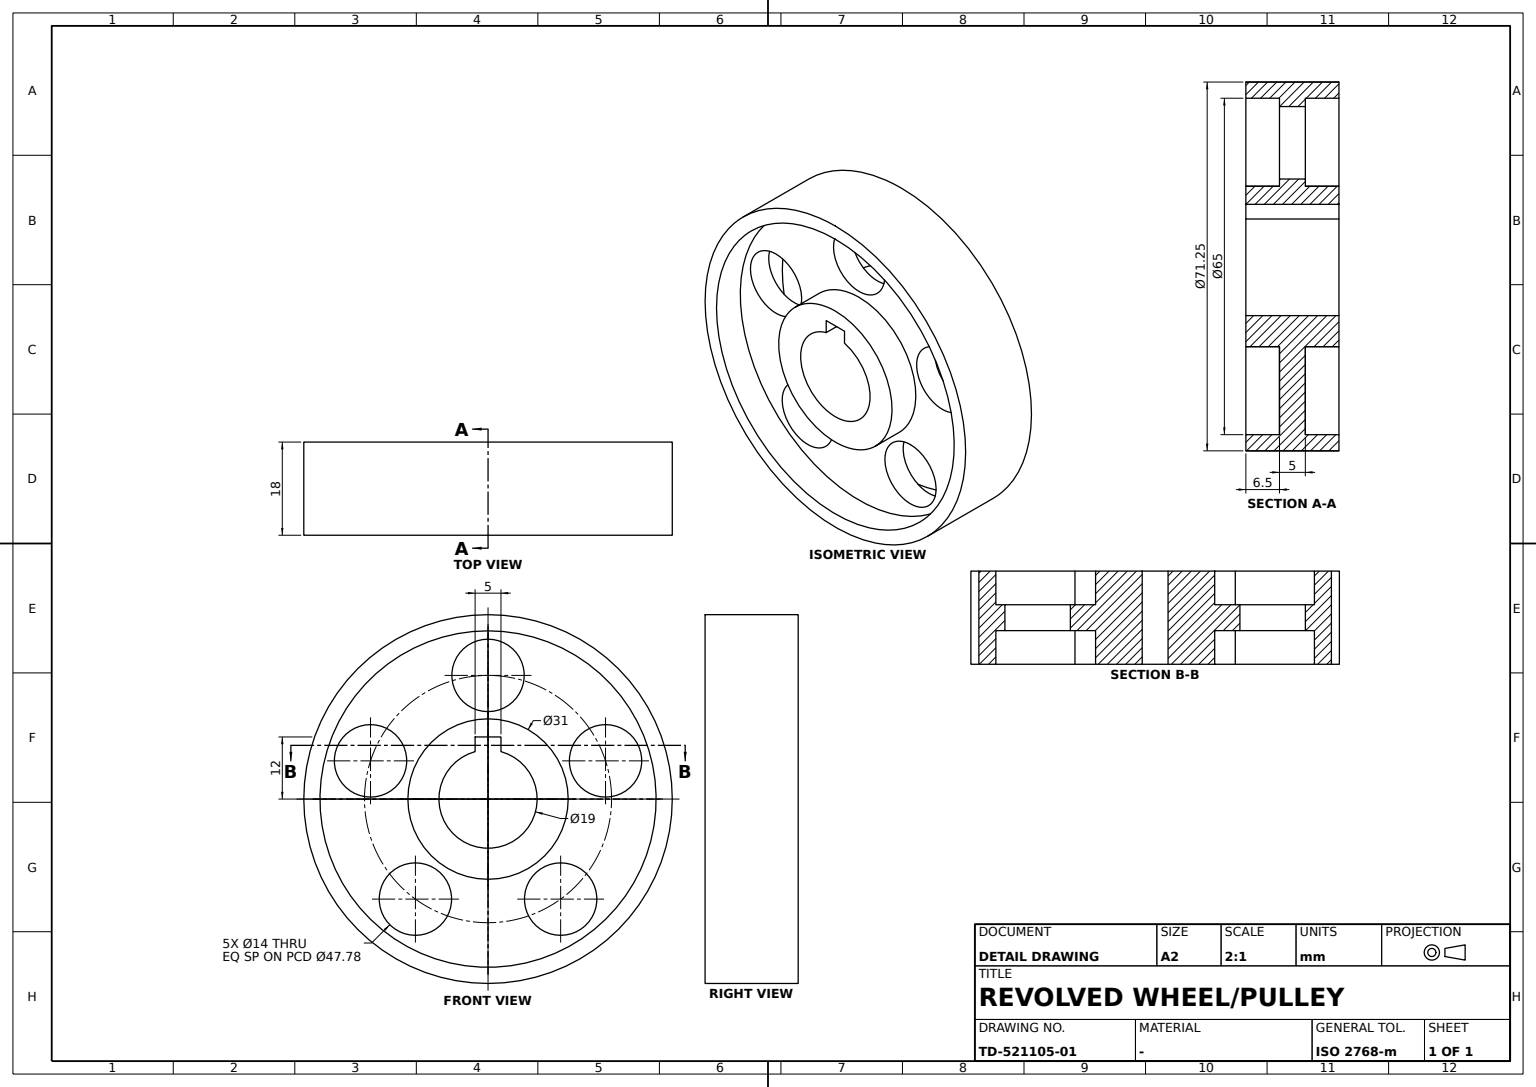
CATIA V5 part; units mm, degrees
sketch "Sketch1" plane through (0, 0, 0) normal (0, 1, 0) x (-1, 0, 0)
  point P0 (0, 9.5)
  line L0 (0, 9.5) -> (-5.7, 9.5)
  line L1 (-5.7, 9.5) -> (-5.7, 15.5)
  line L2 (-5.7, 15.5) -> (0.8, 15.5)
  line L3 (0.8, 15.5) -> (0.8, 32.5)
  line L4 (0.8, 32.5) -> (-5.7, 32.5)
  point P1 (-5.7, 32.5)
  line L5 (-5.7, 32.5) -> (-5.7, 35.625)
  point P2 (-5.7, 35.625)
  line L6 (-5.7, 35.625) -> (12.3, 35.625)
  line L7 (12.3, 35.625) -> (12.3, 32.5)
  point P3 (12.3, 32.5)
  line L8 (12.3, 32.5) -> (5.8, 32.5)
  line L9 (5.8, 32.5) -> (5.8, 15.5)
  point P4 (5.8, 15.5)
  line L10 (5.8, 15.5) -> (12.3, 15.5)
  point P5 (12.3, 15.5)
  line L11 (12.3, 15.5) -> (12.3, 9.5)
  point P6 (12.3, 9.5)
  line L12 (12.3, 9.5) -> (0, 9.5)
  dimension "length L7" = 3.125
  dimension "length L11" = 6
  dimension "distance L1 y axis" = 5.7
  dimension "distance L3 P2" = 6.5
  dimension "distance L3 L9" = 5
  dimension "distance L5 L7" = 18
  dimension "distance L6 x axis" = 35.625
  dimension "distance x axis L12" = 9.5
  constraint coincidence P0 y-axis
  constraint coincidence P1 L1
  constraint coincidence P3 L4
  constraint coincidence P4 L2
  constraint coincidence P5 L7
  constraint coincidence P6 L0
  constraint horizontal L0 x-axis
  constraint horizontal L2 x-axis
  constraint horizontal L4 x-axis
  constraint horizontal L6 x-axis
  constraint horizontal L8 x-axis
  constraint horizontal L10 x-axis
  constraint horizontal L12 x-axis
  constraint vertical L1 y-axis
  constraint vertical L3 y-axis
  constraint vertical L5 y-axis
  constraint vertical L7 y-axis
  constraint vertical L9 y-axis
  constraint vertical L11 y-axis
revolve "Shaft1" add sketch "Sketch1" angle 360 about axis through (0, 0, 0) along (-1, 0, 0)
sketch "Sketch2" plane through (0, 0, 0) normal (1, 0, 0) x (0, 1, 0)
  circle A0 centre (0, 23.89) radius 7
  point P0 (0, 23.89)
  circle A1 centre (-22.7207, 7.3824) radius 7
  circle A2 centre (-14.0422, -19.3274) radius 7
  circle A3 centre (14.0422, -19.3274) radius 7
  circle A4 centre (22.7207, 7.3824) radius 7
  circle A5 centre (0, 0) radius 9.5 construction
  arc A6 (2.5, 9.1652) -> (-2.5, 9.1652) centre (0, 0) ccw
  line L0 (-2.5, 12) -> (2.5, 12)
  line L1 (2.5, 12) -> (2.5, 9.1652)
  line L2 (-2.5, 9.1652) -> (-2.5, 12)
  point P1 (-2.5, 9.1652)
  point P2 (2.5, 9.1652)
  dimension "radius A0" = 7
  dimension "distance x axis P0" = 23.89
  dimension "distance x axis L0" = 12
  dimension "distance L2 y axis" = 2.5
  dimension "distance y axis L1" = 2.5
  constraint coincidence P0 y-axis
  constraint coincidence A5 P1
  constraint coincidence A5 P2
  constraint horizontal L0 x-axis
  constraint vertical L1 y-axis
  constraint vertical L2 y-axis
extrude "Pocket1" cut sketch "Sketch2" along normal mid plane 40
